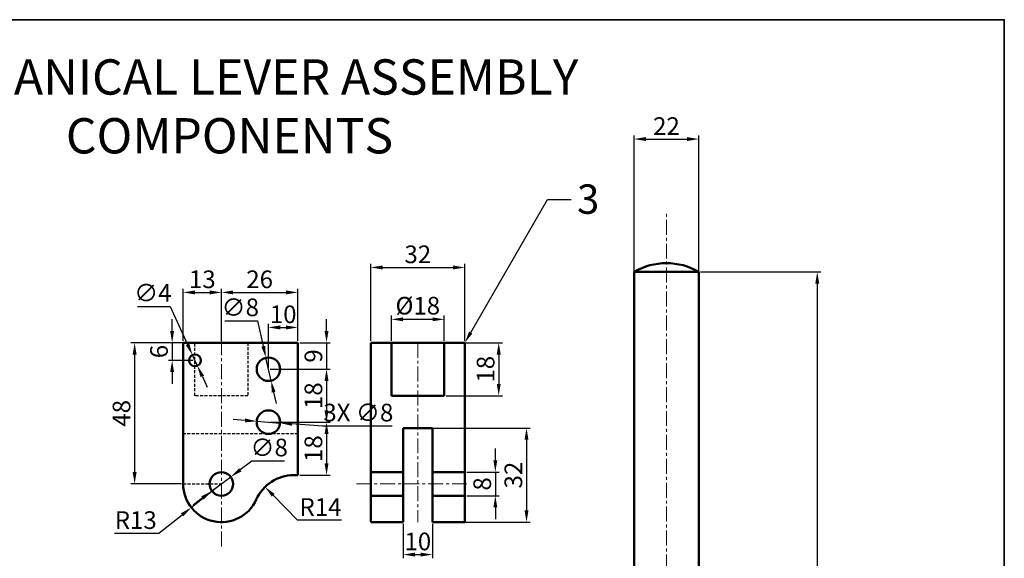
# Model space of a CAD drawing. Units: millimetres. Extents: x 44 to 571, y -292 to 291.
# Tile 4 of 4: x 236 to 571, y 108 to 291. Entities that reach past the tile are written whole.
import ezdxf
from ezdxf import colors
from ezdxf.entities.mleader import LeaderData, LeaderLine
from ezdxf.math import Vec2, Vec3

# ---------------------------------------------------------------- set-up
doc = ezdxf.new("R2010")
doc.units = ezdxf.units.MM
doc.header["$LTSCALE"] = 0.4
doc.linetypes.add('CENTER', pattern=[50.8, 31.75, -6.35, 6.35, -6.35])
doc.linetypes.add('HIDDEN', pattern=[9.525, 6.35, -3.175])
for name, color, linetype, lineweight in [('M-CNTR', 1, 'CENTER', 18), ('M-DIMS', 2, 'Continuous', 25), ('M-HATC', 8, 'Continuous', 18), ('M-HIDN', 3, 'HIDDEN', 25), ('M-OUTL', 7, 'Continuous', 50), ('M-TEXT', 3, 'Continuous', 25), ('M-TTLB', 7, 'Continuous', 35)]:
    doc.layers.add(name, color=color, linetype=linetype, lineweight=lineweight)
doc.styles.get("Standard").update_dxf_attribs({"font": 'arial.ttf'})
doc.dimstyles.new('ISO-25', dxfattribs={"dimtxt": 6, "dimasz": 4, "dimexe": 1.25, "dimexo": 0.625, "dimtad": 1, "dimtoh": 1, "dimdec": 0, "dimtxsty": 'Standard', "dimcen": 2.5, "dimadec": 0, "dimazin": 0, "dimtfac": 1, "dimtdec": 0, "dimtmove": 0, "dimatfit": 3, "dimfxl": 1, "dimarcsym": 0})

# ---------------------------------------------------------------- blocks, each defined once
blk = doc.blocks.new('*D18')
at = {"layer": 'Defpoints', "color": 0, "ltscale": 0.4, "transparency": 16777216}
for p in [(330.38, 186.47), (330.38, 181.27), (320.38, 172.27)]:
    blk.add_point(p, dxfattribs=at)
at = {"layer": 'M-DIMS', "color": 0, "lineweight": -2, "ltscale": 0.4, "transparency": 16777216}
for p, q in [((320.38, 172.9), (320.38, 187.72)), ((330.38, 181.9), (330.38, 187.72)), ((324.38, 186.47), (326.38, 186.47))]:
    blk.add_line(p, q, dxfattribs=at)
at = {"layer": 'M-DIMS', "color": 0, "ltscale": 0.4, "transparency": 16777216}
for points in [[(324.38, 187.14), (324.38, 185.8), (320.38, 186.47)], [(326.38, 187.14), (326.38, 185.8), (330.38, 186.47)]]:
    blk.add_solid(points, dxfattribs=at)
at = {"layer": 'M-DIMS', "color": 0, "ltscale": 0.4, "transparency": 16777216, "insert": (325.38, 190.16), "char_height": 6, "attachment_point": 5}
blk.add_mtext('10', dxfattribs=at)
blk = doc.blocks.new('*D19')
at = {"layer": 'Defpoints', "color": 0, "ltscale": 0.4, "transparency": 16777216}
for p in [(330.38, 198.38), (304.38, 181.27), (330.38, 181.27)]:
    blk.add_point(p, dxfattribs=at)
at = {"layer": 'M-DIMS', "color": 0, "lineweight": -2, "ltscale": 0.4, "transparency": 16777216}
for p, q in [((304.38, 181.9), (304.38, 199.63)), ((308.38, 198.38), (326.38, 198.38)), ((330.38, 181.9), (330.38, 199.63))]:
    blk.add_line(p, q, dxfattribs=at)
at = {"layer": 'M-DIMS', "color": 0, "ltscale": 0.4, "transparency": 16777216}
for points in [[(308.38, 199.05), (308.38, 197.71), (304.38, 198.38)], [(326.38, 199.05), (326.38, 197.71), (330.38, 198.38)]]:
    blk.add_solid(points, dxfattribs=at)
at = {"layer": 'M-DIMS', "color": 0, "ltscale": 0.4, "transparency": 16777216, "insert": (317.38, 202.07), "char_height": 6, "attachment_point": 5}
blk.add_mtext('26', dxfattribs=at)
blk = doc.blocks.new('*D20')
at = {"layer": 'Defpoints', "color": 0, "ltscale": 0.4, "transparency": 16777216}
for p in [(304.38, 198.38), (291.38, 181.27), (304.38, 181.27)]:
    blk.add_point(p, dxfattribs=at)
at = {"layer": 'M-DIMS', "color": 0, "lineweight": -2, "ltscale": 0.4, "transparency": 16777216}
for p, q in [((291.38, 181.9), (291.38, 199.63)), ((295.38, 198.38), (300.38, 198.38)), ((304.38, 181.9), (304.38, 199.63))]:
    blk.add_line(p, q, dxfattribs=at)
at = {"layer": 'M-DIMS', "color": 0, "ltscale": 0.4, "transparency": 16777216}
for points in [[(295.38, 199.05), (295.38, 197.71), (291.38, 198.38)], [(300.38, 199.05), (300.38, 197.71), (304.38, 198.38)]]:
    blk.add_solid(points, dxfattribs=at)
at = {"layer": 'M-DIMS', "color": 0, "ltscale": 0.4, "transparency": 16777216, "insert": (297.88, 202.07), "char_height": 6, "attachment_point": 5}
blk.add_mtext('13', dxfattribs=at)
blk = doc.blocks.new('*D21')
at = {"layer": 'Defpoints', "color": 0, "ltscale": 0.4, "transparency": 16777216}
for p in [(295.38, 181.27), (287.63, 175.27), (295.38, 175.27)]:
    blk.add_point(p, dxfattribs=at)
at = {"layer": 'M-DIMS', "color": 0, "lineweight": -2, "ltscale": 0.4, "transparency": 16777216}
for p, q in [((287.63, 185.27), (287.63, 189.27)), ((294.76, 181.27), (286.38, 181.27)), ((287.63, 181.27), (287.63, 175.27)), ((294.76, 175.27), (286.38, 175.27)), ((287.63, 171.27), (287.63, 167.27))]:
    blk.add_line(p, q, dxfattribs=at)
at = {"layer": 'M-DIMS', "color": 0, "ltscale": 0.4, "transparency": 16777216}
for points in [[(286.96, 185.27), (288.29, 185.27), (287.63, 181.27)], [(286.96, 171.27), (288.29, 171.27), (287.63, 175.27)]]:
    blk.add_solid(points, dxfattribs=at)
at = {"layer": 'M-DIMS', "color": 0, "ltscale": 0.4, "transparency": 16777216, "insert": (283.94, 178.27), "char_height": 6, "attachment_point": 5, "rotation": 90}
blk.add_mtext('6', dxfattribs=at)
blk = doc.blocks.new('*D22')
at = {"layer": 'Defpoints', "color": 0, "ltscale": 0.4, "transparency": 16777216}
for p in [(291.38, 181.27), (274.88, 133.27), (291.38, 133.27)]:
    blk.add_point(p, dxfattribs=at)
at = {"layer": 'M-DIMS', "color": 0, "lineweight": -2, "ltscale": 0.4, "transparency": 16777216}
for p, q in [((290.76, 181.27), (273.63, 181.27)), ((274.88, 177.27), (274.88, 137.27)), ((290.76, 133.27), (273.63, 133.27))]:
    blk.add_line(p, q, dxfattribs=at)
at = {"layer": 'M-DIMS', "color": 0, "ltscale": 0.4, "transparency": 16777216}
for points in [[(274.21, 177.27), (275.55, 177.27), (274.88, 181.27)], [(274.21, 137.27), (275.55, 137.27), (274.88, 133.27)]]:
    blk.add_solid(points, dxfattribs=at)
at = {"layer": 'M-DIMS', "color": 0, "ltscale": 0.4, "transparency": 16777216, "insert": (271.19, 157.27), "char_height": 6, "attachment_point": 5, "rotation": 90}
blk.add_mtext('48', dxfattribs=at)
blk = doc.blocks.new('*D23')
at = {"layer": 'Defpoints', "color": 0, "ltscale": 0.4, "transparency": 16777216}
for p in [(330.38, 181.27), (320.38, 172.27), (340.13, 172.27)]:
    blk.add_point(p, dxfattribs=at)
at = {"layer": 'M-DIMS', "color": 0, "lineweight": -2, "ltscale": 0.4, "transparency": 16777216}
for p, q in [((340.13, 185.27), (340.13, 189.27)), ((331.01, 181.27), (341.38, 181.27)), ((340.13, 181.27), (340.13, 172.27)), ((321.01, 172.27), (341.38, 172.27)), ((340.13, 168.27), (340.13, 164.27))]:
    blk.add_line(p, q, dxfattribs=at)
at = {"layer": 'M-DIMS', "color": 0, "ltscale": 0.4, "transparency": 16777216}
for points in [[(339.46, 185.27), (340.8, 185.27), (340.13, 181.27)], [(339.46, 168.27), (340.8, 168.27), (340.13, 172.27)]]:
    blk.add_solid(points, dxfattribs=at)
at = {"layer": 'M-DIMS', "color": 0, "ltscale": 0.4, "transparency": 16777216, "insert": (336.44, 176.77), "char_height": 6, "attachment_point": 5, "rotation": 90}
blk.add_mtext('9', dxfattribs=at)
blk = doc.blocks.new('*D24')
at = {"layer": 'Defpoints', "color": 0, "ltscale": 0.4, "transparency": 16777216}
for p in [(320.38, 172.27), (320.38, 154.27), (340.13, 154.27)]:
    blk.add_point(p, dxfattribs=at)
at = {"layer": 'M-DIMS', "color": 0, "lineweight": -2, "ltscale": 0.4, "transparency": 16777216}
for p, q in [((321.01, 172.27), (341.38, 172.27)), ((340.13, 168.27), (340.13, 158.27)), ((321.01, 154.27), (341.38, 154.27))]:
    blk.add_line(p, q, dxfattribs=at)
at = {"layer": 'M-DIMS', "color": 0, "ltscale": 0.4, "transparency": 16777216}
for points in [[(339.46, 168.27), (340.8, 168.27), (340.13, 172.27)], [(339.46, 158.27), (340.8, 158.27), (340.13, 154.27)]]:
    blk.add_solid(points, dxfattribs=at)
at = {"layer": 'M-DIMS', "color": 0, "ltscale": 0.4, "transparency": 16777216, "insert": (336.44, 163.27), "char_height": 6, "attachment_point": 5, "rotation": 90}
blk.add_mtext('18', dxfattribs=at)
blk = doc.blocks.new('*D25')
at = {"layer": 'Defpoints', "color": 0, "ltscale": 0.4, "transparency": 16777216}
for p in [(330.38, 154.27), (330.38, 136.27), (340.13, 136.27)]:
    blk.add_point(p, dxfattribs=at)
at = {"layer": 'M-DIMS', "color": 0, "lineweight": -2, "ltscale": 0.4, "transparency": 16777216}
for p, q in [((331.01, 154.27), (341.38, 154.27)), ((340.13, 150.27), (340.13, 140.27)), ((331.01, 136.27), (341.38, 136.27))]:
    blk.add_line(p, q, dxfattribs=at)
at = {"layer": 'M-DIMS', "color": 0, "ltscale": 0.4, "transparency": 16777216}
for points in [[(339.46, 150.27), (340.8, 150.27), (340.13, 154.27)], [(339.46, 140.27), (340.8, 140.27), (340.13, 136.27)]]:
    blk.add_solid(points, dxfattribs=at)
at = {"layer": 'M-DIMS', "color": 0, "ltscale": 0.4, "transparency": 16777216, "insert": (336.44, 145.27), "char_height": 6, "attachment_point": 5, "rotation": 90}
blk.add_mtext('18', dxfattribs=at)
blk = doc.blocks.new('*D26')
at = {"layer": 'Defpoints', "color": 0, "ltscale": 0.4, "transparency": 16777216}
for p in [(371.16, 152.27), (376.16, 120.27), (408.12, 120.27)]:
    blk.add_point(p, dxfattribs=at)
at = {"layer": 'M-DIMS', "color": 0, "lineweight": -2, "ltscale": 0.4, "transparency": 16777216}
for p, q in [((371.78, 152.27), (409.37, 152.27)), ((408.12, 148.27), (408.12, 124.27)), ((376.78, 120.27), (409.37, 120.27))]:
    blk.add_line(p, q, dxfattribs=at)
at = {"layer": 'M-DIMS', "color": 0, "ltscale": 0.4, "transparency": 16777216}
for points in [[(407.45, 148.27), (408.78, 148.27), (408.12, 152.27)], [(407.45, 124.27), (408.78, 124.27), (408.12, 120.27)]]:
    blk.add_solid(points, dxfattribs=at)
at = {"layer": 'M-DIMS', "color": 0, "ltscale": 0.4, "transparency": 16777216, "insert": (404.43, 136.27), "char_height": 6, "attachment_point": 5, "rotation": 90}
blk.add_mtext('32', dxfattribs=at)
blk = doc.blocks.new('*D27')
at = {"layer": 'Defpoints', "color": 0, "ltscale": 0.4, "transparency": 16777216}
for p in [(387.16, 137.27), (387.16, 129.27), (397.52, 129.27)]:
    blk.add_point(p, dxfattribs=at)
at = {"layer": 'M-DIMS', "color": 0, "lineweight": -2, "ltscale": 0.4, "transparency": 16777216}
for p, q in [((397.52, 141.27), (397.52, 145.27)), ((387.78, 137.27), (398.77, 137.27)), ((397.52, 137.27), (397.52, 129.27)), ((387.78, 129.27), (398.77, 129.27)), ((397.52, 125.27), (397.52, 121.27))]:
    blk.add_line(p, q, dxfattribs=at)
at = {"layer": 'M-DIMS', "color": 0, "ltscale": 0.4, "transparency": 16777216}
for points in [[(396.85, 141.27), (398.18, 141.27), (397.52, 137.27)], [(396.85, 125.27), (398.18, 125.27), (397.52, 129.27)]]:
    blk.add_solid(points, dxfattribs=at)
at = {"layer": 'M-DIMS', "color": 0, "ltscale": 0.4, "transparency": 16777216, "insert": (393.83, 133.27), "char_height": 6, "attachment_point": 5, "rotation": 90}
blk.add_mtext('8', dxfattribs=at)
blk = doc.blocks.new('*D28')
at = {"layer": 'Defpoints', "color": 0, "ltscale": 0.4, "transparency": 16777216}
for p in [(380.16, 181.27), (380.16, 163.27), (398.67, 163.27)]:
    blk.add_point(p, dxfattribs=at)
at = {"layer": 'M-DIMS', "color": 0, "lineweight": -2, "ltscale": 0.4, "transparency": 16777216}
for p, q in [((380.78, 181.27), (399.92, 181.27)), ((398.67, 177.27), (398.67, 167.27)), ((380.78, 163.27), (399.92, 163.27))]:
    blk.add_line(p, q, dxfattribs=at)
at = {"layer": 'M-DIMS', "color": 0, "ltscale": 0.4, "transparency": 16777216}
for points in [[(398, 177.27), (399.34, 177.27), (398.67, 181.27)], [(398, 167.27), (399.34, 167.27), (398.67, 163.27)]]:
    blk.add_solid(points, dxfattribs=at)
at = {"layer": 'M-DIMS', "color": 0, "ltscale": 0.4, "transparency": 16777216, "insert": (394.98, 172.27), "char_height": 6, "attachment_point": 5, "rotation": 90}
blk.add_mtext('18', dxfattribs=at)
blk = doc.blocks.new('*D29')
at = {"layer": 'Defpoints', "color": 0, "ltscale": 0.4, "transparency": 16777216}
for p in [(380.16, 189.23), (362.16, 181.27), (380.16, 181.27)]:
    blk.add_point(p, dxfattribs=at)
at = {"layer": 'M-DIMS', "color": 0, "lineweight": -2, "ltscale": 0.4, "transparency": 16777216}
for p, q in [((362.16, 181.9), (362.16, 190.48)), ((366.16, 189.23), (376.16, 189.23)), ((380.16, 181.9), (380.16, 190.48))]:
    blk.add_line(p, q, dxfattribs=at)
at = {"layer": 'M-DIMS', "color": 0, "ltscale": 0.4, "transparency": 16777216}
for points in [[(366.16, 189.9), (366.16, 188.57), (362.16, 189.23)], [(376.16, 189.9), (376.16, 188.57), (380.16, 189.23)]]:
    blk.add_solid(points, dxfattribs=at)
at = {"layer": 'M-DIMS', "color": 0, "ltscale": 0.4, "transparency": 16777216, "insert": (371.16, 193.09), "char_height": 6, "attachment_point": 5}
blk.add_mtext('%%C18', dxfattribs=at)
blk = doc.blocks.new('*D30')
at = {"layer": 'Defpoints', "color": 0, "ltscale": 0.4, "transparency": 16777216}
for p in [(387.16, 206.87), (355.16, 181.27), (387.16, 181.27)]:
    blk.add_point(p, dxfattribs=at)
at = {"layer": 'M-DIMS', "color": 0, "lineweight": -2, "ltscale": 0.4, "transparency": 16777216}
for p, q in [((355.16, 181.9), (355.16, 208.12)), ((387.16, 181.9), (387.16, 208.12)), ((359.16, 206.87), (383.16, 206.87))]:
    blk.add_line(p, q, dxfattribs=at)
at = {"layer": 'M-DIMS', "color": 0, "ltscale": 0.4, "transparency": 16777216}
for points in [[(359.16, 207.53), (359.16, 206.2), (355.16, 206.87)], [(383.16, 207.53), (383.16, 206.2), (387.16, 206.87)]]:
    blk.add_solid(points, dxfattribs=at)
at = {"layer": 'M-DIMS', "color": 0, "ltscale": 0.4, "transparency": 16777216, "insert": (371.16, 210.56), "char_height": 6, "attachment_point": 5}
blk.add_mtext('32', dxfattribs=at)
blk = doc.blocks.new('*D31')
at = {"layer": 'Defpoints', "color": 0, "ltscale": 0.4, "transparency": 16777216}
for p in [(319.5, 176.17), (321.27, 168.37)]:
    blk.add_point(p, dxfattribs=at)
at = {"layer": 'M-DIMS', "color": 0, "lineweight": -2, "ltscale": 0.4, "transparency": 16777216}
for p, q in [((305.56, 188.68), (316.66, 188.68)), ((316.66, 188.68), (318.61, 180.07)), ((321.27, 168.37), (319.5, 176.17)), ((322.15, 164.47), (323.04, 160.57))]:
    blk.add_line(p, q, dxfattribs=at)
at = {"layer": 'M-DIMS', "color": 0, "ltscale": 0.4, "transparency": 16777216}
for points in [[(319.26, 180.22), (317.96, 179.92), (319.5, 176.17)], [(322.8, 164.62), (321.5, 164.32), (321.27, 168.37)]]:
    blk.add_solid(points, dxfattribs=at)
at = {"layer": 'M-DIMS', "color": 0, "ltscale": 0.4, "transparency": 16777216, "insert": (310.8, 192.53), "char_height": 6, "attachment_point": 5}
blk.add_mtext('∅8', dxfattribs=at)
blk = doc.blocks.new('*D32')
at = {"layer": 'Defpoints', "color": 0, "ltscale": 0.4, "transparency": 16777216}
for p in [(294.54, 177.09), (296.22, 173.46)]:
    blk.add_point(p, dxfattribs=at)
at = {"layer": 'M-DIMS', "color": 0, "lineweight": -2, "ltscale": 0.4, "transparency": 16777216}
for p, q in [((275.86, 193.58), (286.92, 193.58)), ((286.92, 193.58), (292.87, 180.72)), ((296.22, 173.46), (294.54, 177.09)), ((297.9, 169.82), (299.58, 166.19))]:
    blk.add_line(p, q, dxfattribs=at)
at = {"layer": 'M-DIMS', "color": 0, "ltscale": 0.4, "transparency": 16777216}
for points in [[(293.47, 181), (292.26, 180.44), (294.54, 177.09)], [(298.51, 170.1), (297.29, 169.55), (296.22, 173.46)]]:
    blk.add_solid(points, dxfattribs=at)
at = {"layer": 'M-DIMS', "color": 0, "ltscale": 0.4, "transparency": 16777216, "insert": (281.08, 197.44), "char_height": 6, "attachment_point": 5}
blk.add_mtext('∅4', dxfattribs=at)
blk = doc.blocks.new('*D33')
at = {"layer": 'Defpoints', "color": 0, "ltscale": 0.4, "transparency": 16777216}
for p in [(319.21, 132.24), (329.04, 122.27)]:
    blk.add_point(p, dxfattribs=at)
at = {"layer": 'M-DIMS', "color": 0, "lineweight": -2, "ltscale": 0.4, "transparency": 16777216}
for p, q in [((330.29, 121), (322.02, 129.39)), ((345.23, 121), (330.29, 121))]:
    blk.add_line(p, q, dxfattribs=at)
at = {"layer": 'M-DIMS', "color": 0, "ltscale": 0.4, "transparency": 16777216}
blk.add_solid([(322.49, 129.86), (321.54, 128.92), (319.21, 132.24)], dxfattribs=at)
at = {"layer": 'M-DIMS', "color": 0, "ltscale": 0.4, "transparency": 16777216, "insert": (338.07, 124.64), "char_height": 6, "attachment_point": 5}
blk.add_mtext('R14', dxfattribs=at)
blk = doc.blocks.new('*D34')
at = {"layer": 'Defpoints', "color": 0, "ltscale": 0.4, "transparency": 16777216}
for p in [(304.38, 133.27), (294.16, 125.24)]:
    blk.add_point(p, dxfattribs=at)
at = {"layer": 'M-DIMS', "color": 0, "lineweight": -2, "ltscale": 0.4, "transparency": 16777216}
for p, q in [((304.38, 133.27), (294.16, 125.24)), ((283.06, 116.5), (291.02, 122.76)), ((268.09, 116.5), (283.06, 116.5))]:
    blk.add_line(p, q, dxfattribs=at)
at = {"layer": 'M-DIMS', "color": 0, "ltscale": 0.4, "transparency": 16777216}
blk.add_solid([(290.61, 123.29), (291.43, 122.24), (294.16, 125.24)], dxfattribs=at)
at = {"layer": 'M-DIMS', "color": 0, "ltscale": 0.4, "transparency": 16777216, "insert": (275.26, 120.19), "char_height": 6, "attachment_point": 5}
blk.add_mtext('R13', dxfattribs=at)
blk = doc.blocks.new('*D35')
at = {"layer": 'Defpoints', "color": 0, "ltscale": 0.4, "transparency": 16777216}
for p in [(307.59, 135.66), (301.18, 130.88)]:
    blk.add_point(p, dxfattribs=at)
at = {"layer": 'M-DIMS', "color": 0, "lineweight": -2, "ltscale": 0.4, "transparency": 16777216}
for p, q in [((314.77, 141.01), (310.8, 138.05)), ((325.87, 141.01), (314.77, 141.01)), ((301.18, 130.88), (307.59, 135.66)), ((297.97, 128.49), (294.76, 126.1))]:
    blk.add_line(p, q, dxfattribs=at)
at = {"layer": 'M-DIMS', "color": 0, "ltscale": 0.4, "transparency": 16777216}
for points in [[(310.4, 138.59), (311.2, 137.52), (307.59, 135.66)], [(297.57, 129.03), (298.37, 127.96), (301.18, 130.88)]]:
    blk.add_solid(points, dxfattribs=at)
at = {"layer": 'M-DIMS', "color": 0, "ltscale": 0.4, "transparency": 16777216, "insert": (320.63, 144.87), "char_height": 6, "attachment_point": 5}
blk.add_mtext('∅8', dxfattribs=at)
blk = doc.blocks.new('*D36')
at = {"layer": 'Defpoints', "color": 0, "ltscale": 0.4, "transparency": 16777216}
for p in [(366.16, 120.27), (376.16, 120.27), (376.16, 109.24)]:
    blk.add_point(p, dxfattribs=at)
at = {"layer": 'M-DIMS', "color": 0, "lineweight": -2, "ltscale": 0.4, "transparency": 16777216}
for p, q in [((366.16, 119.65), (366.16, 107.99)), ((376.16, 119.65), (376.16, 107.99)), ((370.16, 109.24), (372.16, 109.24))]:
    blk.add_line(p, q, dxfattribs=at)
at = {"layer": 'M-DIMS', "color": 0, "ltscale": 0.4, "transparency": 16777216}
for points in [[(370.16, 109.91), (370.16, 108.58), (366.16, 109.24)], [(372.16, 109.91), (372.16, 108.58), (376.16, 109.24)]]:
    blk.add_solid(points, dxfattribs=at)
at = {"layer": 'M-DIMS', "color": 0, "ltscale": 0.4, "transparency": 16777216, "insert": (371.16, 112.93), "char_height": 6, "attachment_point": 5}
blk.add_mtext('10', dxfattribs=at)
blk = doc.blocks.new('*D53')
at = {"layer": 'Defpoints', "color": 0, "ltscale": 0.4, "transparency": 16777216}
for p in [(466.7, 205.39), (466.7, -74.61), (506.97, -74.61)]:
    blk.add_point(p, dxfattribs=at)
at = {"layer": 'M-DIMS', "color": 0, "lineweight": -2, "ltscale": 0.4, "transparency": 16777216}
for p, q in [((467.32, 205.39), (508.22, 205.39)), ((506.97, 201.39), (506.97, -70.61)), ((467.32, -74.61), (508.22, -74.61))]:
    blk.add_line(p, q, dxfattribs=at)
at = {"layer": 'M-DIMS', "color": 0, "ltscale": 0.4, "transparency": 16777216}
for points in [[(506.3, 201.39), (507.64, 201.39), (506.97, 205.39)], [(506.3, -70.61), (507.64, -70.61), (506.97, -74.61)]]:
    blk.add_solid(points, dxfattribs=at)
at = {"layer": 'M-DIMS', "color": 0, "ltscale": 0.4, "transparency": 16777216, "insert": (503.28, 65.39), "char_height": 6, "attachment_point": 5, "rotation": 90}
blk.add_mtext('280', dxfattribs=at)
blk = doc.blocks.new('*D76')
at = {"layer": 'Defpoints', "color": 0, "ltscale": 0.4, "transparency": 16777216}
for p in [(466.7, 250.52), (444.7, 205.39), (466.7, 205.39)]:
    blk.add_point(p, dxfattribs=at)
at = {"layer": 'M-DIMS', "color": 0, "lineweight": -2, "ltscale": 0.4, "transparency": 16777216}
for p, q in [((444.7, 206.01), (444.7, 251.77)), ((466.7, 206.01), (466.7, 251.77)), ((448.7, 250.52), (462.7, 250.52))]:
    blk.add_line(p, q, dxfattribs=at)
at = {"layer": 'M-DIMS', "color": 0, "ltscale": 0.4, "transparency": 16777216}
for points in [[(448.7, 251.19), (448.7, 249.85), (444.7, 250.52)], [(462.7, 251.19), (462.7, 249.85), (466.7, 250.52)]]:
    blk.add_solid(points, dxfattribs=at)
at = {"layer": 'M-DIMS', "color": 0, "ltscale": 0.4, "transparency": 16777216, "insert": (455.7, 254.16), "char_height": 6, "attachment_point": 5}
blk.add_mtext('22', dxfattribs=at)
blk = doc.blocks.new('*D77')
at = {"layer": 'Defpoints', "color": 0, "ltscale": 0.4, "transparency": 16777216}
for p in [(466.7, 250.52), (444.7, -228.61), (466.7, -228.61)]:
    blk.add_point(p, dxfattribs=at)
at = {"layer": 'M-DIMS', "color": 0, "lineweight": -2, "ltscale": 0.4, "transparency": 16777216}
for p, q in [((444.7, -227.99), (444.7, 251.77)), ((466.7, -227.99), (466.7, 251.77)), ((448.7, 250.52), (462.7, 250.52))]:
    blk.add_line(p, q, dxfattribs=at)
at = {"layer": 'M-DIMS', "color": 0, "ltscale": 0.4, "transparency": 16777216}
for points in [[(448.7, 251.19), (448.7, 249.85), (444.7, 250.52)], [(462.7, 251.19), (462.7, 249.85), (466.7, 250.52)]]:
    blk.add_solid(points, dxfattribs=at)
at = {"layer": 'M-DIMS', "color": 0, "ltscale": 0.4, "transparency": 16777216, "insert": (455.7, 254.16), "char_height": 6, "attachment_point": 5}
blk.add_mtext('22', dxfattribs=at)
blk = doc.blocks.new('*D84')
at = {"layer": 'Defpoints', "color": 0, "ltscale": 0.4, "transparency": 16777216}
for p in [(316.39, 154.57), (324.37, 153.97)]:
    blk.add_point(p, dxfattribs=at)
at = {"layer": 'M-DIMS', "color": 0, "lineweight": -2, "ltscale": 0.4, "transparency": 16777216}
for p, q in [((312.41, 154.87), (308.42, 155.17)), ((316.39, 154.57), (324.37, 153.97)), ((338.79, 152.89), (328.36, 153.67)), ((362.46, 152.89), (338.79, 152.89))]:
    blk.add_line(p, q, dxfattribs=at)
at = {"layer": 'M-DIMS', "color": 0, "ltscale": 0.4, "transparency": 16777216}
for points in [[(312.45, 155.53), (312.36, 154.2), (316.39, 154.57)], [(328.41, 154.34), (328.31, 153.01), (324.37, 153.97)]]:
    blk.add_solid(points, dxfattribs=at)
at = {"layer": 'M-DIMS', "color": 0, "ltscale": 0.4, "transparency": 16777216, "insert": (350.94, 156.75), "char_height": 6, "attachment_point": 5}
blk.add_mtext('3X ∅8', dxfattribs=at)

msp = doc.modelspace()

# ---------------------------------------------------------------- hatches: boundary and pattern name
at = {"layer": 'M-HATC', "ltscale": 0.4}
h = msp.add_hatch(dxfattribs=at)
h.set_pattern_fill('ANSI31', color=256, scale=0.4)
h.paths.add_polyline_path([(466.6963, 51.668), (466.6963, 51.668, 0.41365763), (455.6963, 51.668, 0.41365763)])
h.paths.add_polyline_path([(444.6963, 91.3959, 0.41365763), (455.6963, 91.3959, 0.41365763)])
h.paths.add_polyline_path([(171.2864, 238.6681), (441.8676, 238.6681), (441.8676, 283.6094), (171.2864, 283.6094)], flags=9)

# ---------------------------------------------------------------- linework, layer by layer
at = {"layer": 'M-CNTR', "ltscale": 0.4}
for p, q in [((455.6963, -74.6115), (455.6963, 225.3706)), ((304.3826, 112.0119), (304.3826, 195.716)), ((371.1573, 181.2712), (371.1573, 120.2712)), ((350.2734, 133.2712), (388.6496, 133.2712))]:
    msp.add_line(p, q, dxfattribs=at)
at = {"layer": 'M-HIDN', "ltscale": 0.4}
for p, q in [((295.3826, 163.2712), (295.3826, 181.2712)), ((313.3826, 181.2712), (313.3826, 163.2712)), ((313.3826, 163.2712), (295.3826, 163.2712)), ((330.3826, 150.2712), (291.3826, 150.2712)), ((291.3826, 133.2712), (304.3826, 133.2712))]:
    msp.add_line(p, q, dxfattribs=at)
at = {"layer": 'M-OUTL', "ltscale": 0.4}
for p, q in [((444.6963, 205.3885), (466.6963, 205.3885)), ((444.6963, 91.3959), (444.6963, 205.3885)), ((466.6963, 205.3885), (466.6963, 91.3959)), ((291.3826, 181.2712), (291.3826, 133.2712)), ((291.3826, 181.2712), (330.3826, 181.2712)), ((330.3826, 181.2712), (330.3826, 136.2712)), ((355.1573, 181.2712), (387.1573, 181.2712)), ((355.1573, 120.2712), (355.1573, 181.2712)), ((362.1573, 163.2712), (362.1573, 181.2712)), ((380.1573, 181.2712), (380.1573, 163.2712)), ((387.1573, 181.2712), (387.1573, 120.2712)), ((380.1573, 163.2712), (362.1573, 163.2712)), ((371.1573, 152.2712), (366.1573, 152.2712)), ((366.1573, 152.2712), (366.1573, 120.2712)), ((371.1573, 152.2712), (376.1573, 152.2712)), ((376.1573, 152.2712), (376.1573, 120.2712)), ((355.1573, 137.2712), (366.1573, 137.2712)), ((376.1573, 137.2712), (387.1573, 137.2712)), ((330.3826, 136.2712), (329.0403, 136.2712)), ((355.1573, 129.2712), (366.1573, 129.2712)), ((376.1573, 129.2712), (387.1573, 129.2712)), ((366.1573, 120.2712), (355.1573, 120.2712)), ((387.1573, 120.2712), (376.1573, 120.2712))]:
    msp.add_line(p, q, dxfattribs=at)
for centre, radius in [((295.3826, 175.2712), 2), ((320.3826, 172.2712), 4), ((320.3826, 154.2712), 4), ((304.3826, 133.2712), 4)]:
    msp.add_circle(centre, radius, dxfattribs=at)
for centre, radius, start, end in [((455.6963, 186.3359), 22, 60, 120), ((329.0403, 122.2712), 14, 90, 155.957924), ((304.3826, 133.2712), 13, 180, 335.957924)]:
    msp.add_arc(centre, radius, start, end, dxfattribs=at)
at = {"layer": 'M-TTLB', "ltscale": 0.4}
msp.add_lwpolyline([(44.037, 291.1069), (570.566, 291.1069), (570.566, -292.0762), (44.037, -292.0762)], close=True, dxfattribs=at)

# ---------------------------------------------------------------- texts
at = {"layer": 'M-TTLB', "ltscale": 0.4, "insert": (142.2261, 277.638), "char_height": 12, "attachment_point": 1}
msp.add_mtext_dynamic_manual_height_columns('\\pxqc;MECHANICAL LEVER ASSEMBLY COMPONENTS', width=329.81502, gutter_width=12.5, heights=[0], dxfattribs=at)

# ---------------------------------------------------------------- dimensions: what is measured, and where the dimension line sits
at = {"layer": 'M-DIMS', "ltscale": 0.4}
for base, p1, p2, override, picture, middle in [((466.6963, 250.5206), (444.6963, 205.3885), (466.6963, 205.3885), {"dimdec": 0, "dimlfac": 1, "dimrnd": 0, "dimzin": 0, "dimdsep": 46, "dimlunit": 2}, '*D76', (455.6963, 254.1579)), ((466.6963, 250.5206), (444.6963, -228.6115), (466.6963, -228.6115), {"dimdec": 0, "dimlfac": 1, "dimrnd": 0, "dimzin": 0, "dimdsep": 46, "dimlunit": 2}, '*D77', (455.6963, 254.1579)), ((387.1573, 206.8672), (355.1573, 181.2712), (387.1573, 181.2712), {"dimclrd": 0, "dimclre": 0, "dimclrt": 0}, '*D30', (371.1573, 210.5577)), ((304.3826, 198.3799), (291.3826, 181.2712), (304.3826, 181.2712), {"dimclrd": 0, "dimclre": 0, "dimclrt": 0}, '*D20', (297.8826, 202.0704)), ((330.3826, 198.3799), (304.3826, 181.2712), (330.3826, 181.2712), {"dimclrd": 0, "dimclre": 0, "dimclrt": 0}, '*D19', (317.3826, 202.0683)), ((330.3826, 186.4716), (320.3826, 172.2712), (330.3826, 181.2712), {"dimclrd": 0, "dimclre": 0, "dimclrt": 0}, '*D18', (325.3826, 190.1601)), ((376.1573, 109.2444), (366.1573, 120.2712), (376.1573, 120.2712), {"dimclrd": 0, "dimclre": 0, "dimclrt": 0}, '*D36', (371.1573, 112.9329))]:
    dim = msp.add_linear_dim(base=base, p1=p1, p2=p2, dimstyle='ISO-25', override=override, dxfattribs=at)
    dim.commit()
    dim.dimension.update_dxf_attribs({"geometry": picture, "text_midpoint": middle})
for base, p1, p2, picture, middle in [((506.9684, -74.6115), (466.6963, 205.3885), (466.6963, -74.6115), '*D53', (503.2799, 65.3885)), ((287.6257, 175.2712), (295.3826, 181.2712), (295.3826, 175.2712), '*D21', (283.9373, 178.2712)), ((274.8788, 133.2712), (291.3826, 181.2712), (291.3826, 133.2712), '*D22', (271.1903, 157.2712)), ((398.6709, 163.2712), (380.1573, 181.2712), (380.1573, 163.2712), '*D28', (394.9825, 172.2712)), ((340.1286, 154.2712), (320.3826, 172.2712), (320.3826, 154.2712), '*D24', (336.4401, 163.2712)), ((340.1286, 136.2712), (330.3826, 154.2712), (330.3826, 136.2712), '*D25', (336.4401, 145.2712)), ((408.1164, 120.2712), (371.1573, 152.2712), (376.1573, 120.2712), '*D26', (404.426, 136.2712)), ((397.5171, 129.2712), (387.1573, 137.2712), (387.1573, 129.2712), '*D27', (393.8287, 133.2712))]:
    dim = msp.add_linear_dim(base=base, p1=p1, p2=p2, angle=90, dimstyle='ISO-25', override={"dimclrd": 0, "dimclre": 0, "dimclrt": 0}, dxfattribs=at)
    dim.commit()
    dim.dimension.update_dxf_attribs({"geometry": picture, "text_midpoint": middle})
for p1, p2, picture, middle in [((296.2218, 173.4557), (294.5435, 177.0866), '*D32', (281.0763, 193.5813)), ((321.2683, 168.3704), (319.497, 176.1719), '*D31', (310.7961, 188.6772)), ((301.1754, 130.8809), (307.5899, 135.6614), '*D35', (320.6316, 141.0124))]:
    dim = msp.add_diameter_dim_2p(p1=p1, p2=p2, dimstyle='ISO-25', override={"dimclrd": 0, "dimclre": 0, "dimclrt": 0}, dxfattribs=at)
    dim.commit()
    dim.dimension.update_dxf_attribs({"geometry": picture, "text_midpoint": middle, "dimtype": 163})
dim = msp.add_linear_dim(base=(380.1573, 189.2345), p1=(362.1573, 181.2712), p2=(380.1573, 181.2712), text='%%C<>', dimstyle='ISO-25', override={"dimclrd": 0, "dimclre": 0, "dimclrt": 0}, dxfattribs=at)
dim.commit()
dim.dimension.update_dxf_attribs({"geometry": '*D29', "text_midpoint": (371.1573, 193.0908)})
dim = msp.add_linear_dim(base=(340.1286, 172.2712), p1=(330.3826, 181.2712), p2=(320.3826, 172.2712), angle=90, dimstyle='ISO-25', override={"dimclrd": 0, "dimclre": 0, "dimclrt": 0}, dxfattribs=at)
dim.commit()
dim.dimension.update_dxf_attribs({"geometry": '*D23', "text_midpoint": (340.1286, 176.7712), "dimtype": 160})
dim = msp.add_diameter_dim_2p(p1=(316.3938, 154.5701), p2=(324.3715, 153.9722), text='3X <>', dimstyle='ISO-25', override={"dimdec": 0, "dimlfac": 1, "dimrnd": 0, "dimzin": 0, "dimdsep": 46, "dimlunit": 2}, dxfattribs=at)
dim.commit()
dim.dimension.update_dxf_attribs({"geometry": '*D84', "text_midpoint": (338.7935, 152.8911), "dimtype": 163})
dim = msp.add_radius_dim(center=(304.3826, 133.2712), mpoint=(294.164, 125.235), dimstyle='ISO-25', override={"dimclrd": 0, "dimclre": 0, "dimclrt": 0}, dxfattribs=at)
dim.commit()
dim.dimension.update_dxf_attribs({"geometry": '*D34', "text_midpoint": (275.2629, 120.1903)})
dim = msp.add_radius_dim(center=(329.0403, 122.2712), mpoint=(319.2082, 132.2375), dimstyle='ISO-25', override={"dimclrd": 0, "dimclre": 0, "dimclrt": 0}, dxfattribs=at)
dim.commit()
dim.dimension.update_dxf_attribs({"geometry": '*D33', "text_midpoint": (338.0724, 121.0031), "dimtype": 164})

# ---------------------------------------------------------------- leaders
at = {"layer": 'M-TEXT', "ltscale": 0.4}
ml = msp.add_multileader_mtext('Standard', dxfattribs=at)
ml.set_content('3', color=256)
ml.set_leader_properties()
ml.build(insert=Vec2(0, 0))
ctx = ml.context
ctx.base_point, ctx.char_height, ctx.plane_origin = Vec3(423.2943, 230.0058), 10, Vec3(387.1573, 181.2712)
notes = []
notes.append((ctx, [(0, (1, 1, 0), (415.2943, 230.0058), (1, 0), 8, [(0, [(387.1573, 181.2712)], 0, [])])]))
ctx.mtext.insert, ctx.mtext.flow_direction = Vec3(425.2943, 235.0944), 5
for ctx, leaders in notes:
    for number, flags, end, landing, length, lines in leaders:
        leader = LeaderData()
        leader.index, (leader.has_last_leader_line, leader.has_dogleg_vector, leader.attachment_direction) = number, flags
        leader.last_leader_point, leader.dogleg_vector, leader.dogleg_length = Vec3(end), Vec3(landing), length
        for number, points, colour, breaks in lines:
            line = LeaderLine()
            line.index, line.vertices, line.color, line.breaks = number, Vec3.list(points), colors.encode_raw_color(colour), breaks
            leader.lines.append(line)
        ctx.leaders.append(leader)

doc.saveas('drawing.dxf')
